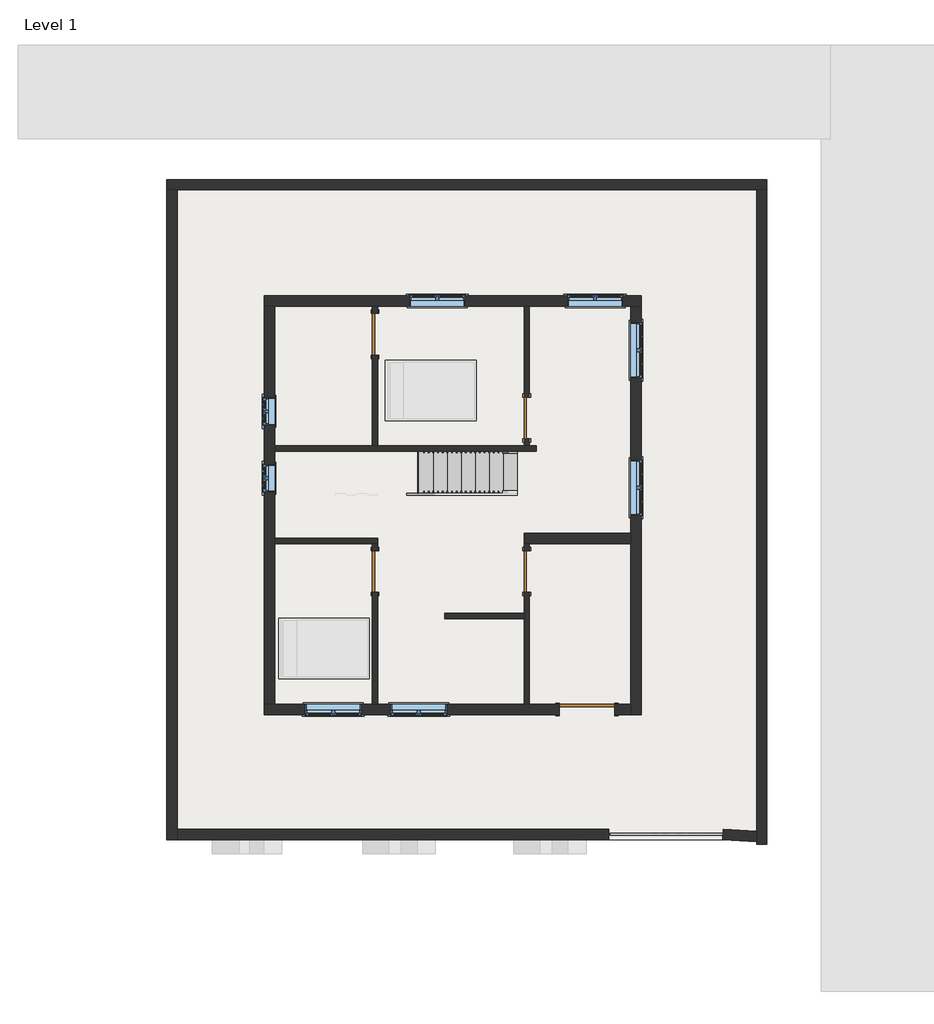
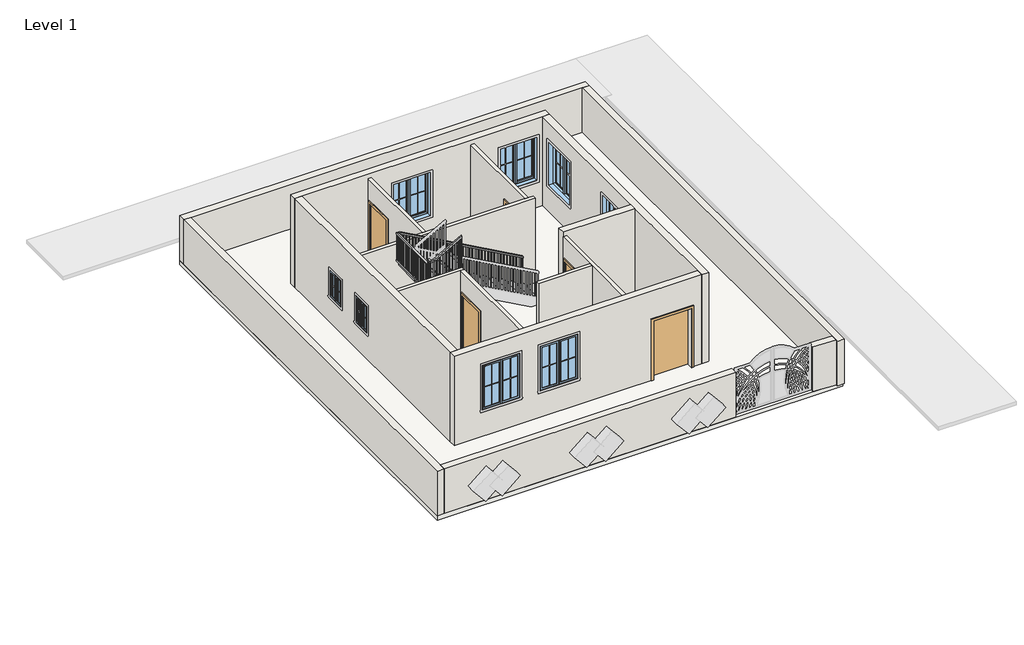
# One storey, part 1 of 2: 17 walls, 8 windows, 5 doors, 1 railing, 1 slab, 1 stair flight.
"""IFC4 building model written with IfcOpenShell, lengths in millimetres."""

from ifc_helpers import new_model, si_unit, frame, origin, origin_with_axes, place, context, project, spatial, polyline, outline, extrude, faceted_brep, transform, mapped, element, save
from components import door_e5f9f3c4, door_305aa2a5, door_48acaae4, stair_flight_91c59d30, window_c417fced, window_8377141f

model = new_model("IFC4")

# Units and contexts
model_context = context("Model", 3, world=origin())
ifc_project = project(units=[si_unit("LENGTHUNIT", "METRE", prefix="MILLI")], contexts=[model_context])

# Site, building, storey
site = spatial("IfcSite", under=ifc_project)
building = spatial("IfcBuilding", under=site)
storey = spatial("IfcBuildingStorey", under=building, Name="Level 1", Elevation=0.0)

# Doors
placement = place(None, origin())
door_shape = door_e5f9f3c4(model_context)
element("IfcDoor", 1, ObjectType="Single-Flush : 36\" x 84\"", at=placement, inside=storey, context=model_context, shape_type="MappedRepresentation", body=[
    mapped(door_shape, transform((3689.35, 13938.7372886, 0.0), x_axis=(0.0, 1.0, 0.0), y_axis=(-1.0, 0.0, 0.0), z_axis=(0.0, 0.0, 1.0))),
])
door_2_shape = door_305aa2a5(model_context)
element("IfcDoor", 2, ObjectType="Single-Flush : 36\" x 84\"", at=placement, inside=storey, context=model_context, shape_type="MappedRepresentation", body=[
    mapped(door_2_shape, transform((7004.05, 12109.9372886, 0.0), x_axis=(0.0, -1.0, 0.0), y_axis=(1.0, 0.0, 0.0), z_axis=(0.0, 0.0, 1.0))),
])
element("IfcDoor", 3, ObjectType="Single-Flush : 36\" x 84\"", at=placement, inside=storey, context=model_context, shape_type="MappedRepresentation", body=[
    mapped(door_2_shape, transform((3689.3519847, 8757.1372886, 0.0), x_axis=(0.0, -1.0, 0.0), y_axis=(1.0, 0.0, 0.0), z_axis=(0.0, 0.0, 1.0))),
])
element("IfcDoor", 4, ObjectType="Single-Flush : 36\" x 84\"", at=placement, inside=storey, context=model_context, shape_type="MappedRepresentation", body=[
    mapped(door_2_shape, transform((7004.05, 8757.1372886, 0.0), x_axis=(0.0, -1.0, 0.0), y_axis=(1.0, 0.0, 0.0), z_axis=(0.0, 0.0, 1.0))),
])
door_3_shape = door_48acaae4(model_context)
element("IfcDoor", 5, ObjectType="Single-Flush : 48\" x 80\"", at=placement, inside=storey, context=model_context, shape_type="MappedRepresentation", body=[
    mapped(door_3_shape, transform((8318.5, 5747.2372886, 0.0), x_axis=(1.0, 0.0, 0.0), y_axis=(0.0, 1.0, 0.0), z_axis=(0.0, 0.0, 1.0))),
])

# Railing
element("IfcRailing", 6, ObjectType="Handrail - Rectangular", at=placement, inside=storey, context=model_context, shape_type="SolidModel", body=[
    faceted_brep([(6794.5, 11335.2372886, 1083.7333333), (6794.5, 11335.2372886, 1025.620221), (6794.5, 11386.0372886, 1025.620221), (6794.5, 11386.0372886, 1083.7333333), (2832.1, 11335.2372886, 3285.0666667), (2818.9363978, 11335.2372886, 3234.2666667), (2818.9363978, 11386.0372886, 3234.2666667), (2832.1, 11386.0372886, 3285.0666667), (2768.6, 11335.2372886, 3285.0666667), (2768.6, 11335.2372886, 3234.2666667), (2717.8, 11386.0372886, 3234.2666667), (2717.8, 11386.0372886, 3285.0666667), (2768.6, 9608.0372886, 3285.0666667), (2768.6, 9557.2372886, 3234.2666667), (2717.8, 9557.2372886, 3234.2666667), (2717.8, 9608.0372886, 3285.0666667), (2768.6, 9608.0372886, 3461.4555402), (2768.6, 9557.2372886, 3410.6555402), (2717.8, 9557.2372886, 3410.6555402), (2717.8, 9608.0372886, 3461.4555402), (2768.6, 9531.8372886, 3461.4555402), (2768.6, 9531.8372886, 3410.6555402), (2717.8, 9481.0372886, 3410.6555402), (2717.8, 9481.0372886, 3461.4555402), (2844.8, 9531.8372886, 3461.4555402), (2857.9635773, 9531.8372886, 3410.6555402), (2857.9635773, 9481.0372886, 3410.6555402), (2844.8, 9481.0372886, 3461.4555402), (3746.5019847, 9531.8372886, 3962.4), (3746.5019847, 9481.0372886, 3962.4), (3746.5019847, 9481.0372886, 3904.2869174), (3746.5019847, 9531.8372886, 3904.2869174)], [[[0, 1, 2, 3]], [[1, 0, 4, 5]], [[2, 1, 5, 6]], [[3, 2, 6, 7]], [[0, 3, 7, 4]], [[5, 4, 8, 9]], [[6, 5, 9, 10]], [[7, 6, 10, 11]], [[4, 7, 11, 8]], [[9, 8, 12, 13]], [[10, 9, 13, 14]], [[11, 10, 14, 15]], [[8, 11, 15, 12]], [[13, 12, 16, 17]], [[14, 13, 17, 18]], [[15, 14, 18, 19]], [[12, 15, 19, 16]], [[17, 16, 20, 21]], [[18, 17, 21, 22]], [[19, 18, 22, 23]], [[16, 19, 23, 20]], [[21, 20, 24, 25]], [[22, 21, 25, 26]], [[23, 22, 26, 27]], [[20, 23, 27, 24]], [[28, 29, 30, 31]], [[25, 24, 28, 31]], [[26, 25, 31, 30]], [[27, 26, 30, 29]], [[24, 27, 29, 28]]]),
    extrude(outline(polyline([(3860.1894234, 3667.125), (3849.606113, 3648.075), (2878.6666667, 3648.075), (2878.6666667, 3667.125), (3860.1894234, 3667.125)])), frame((0.0, 9496.9122886, 0.0), z_axis=(0.0, 1.0, 0.0), x_axis=(0.0, 0.0, 1.0)), (0.0, 0.0, 1.0), 19.05),
    extrude(outline(polyline([(3803.7451014, 3565.525), (3793.1617911, 3546.475), (2878.6666667, 3546.475), (2878.6666667, 3565.525), (3803.7451014, 3565.525)])), frame((0.0, 9496.9122886, 0.0), z_axis=(0.0, 1.0, 0.0), x_axis=(0.0, 0.0, 1.0)), (0.0, 0.0, 1.0), 19.05),
    extrude(outline(polyline([(3747.3007795, 3463.925), (3736.7174691, 3444.875), (2878.6666667, 3444.875), (2878.6666667, 3463.925), (3747.3007795, 3463.925)])), frame((0.0, 9496.9122886, 0.0), z_axis=(0.0, 1.0, 0.0), x_axis=(0.0, 0.0, 1.0)), (0.0, 0.0, 1.0), 19.05),
    extrude(outline(polyline([(3690.85609, 3362.325), (3680.2727797, 3343.275), (2709.3333333, 3343.275), (2709.3333333, 3362.325), (3690.85609, 3362.325)])), frame((0.0, 9496.9122886, 0.0), z_axis=(0.0, 1.0, 0.0), x_axis=(0.0, 0.0, 1.0)), (0.0, 0.0, 1.0), 19.05),
    extrude(outline(polyline([(3634.4117681, 3260.725), (3623.8284577, 3241.675), (2709.3333333, 3241.675), (2709.3333333, 3260.725), (3634.4117681, 3260.725)])), frame((0.0, 9496.9122886, 0.0), z_axis=(0.0, 1.0, 0.0), x_axis=(0.0, 0.0, 1.0)), (0.0, 0.0, 1.0), 19.05),
    extrude(outline(polyline([(3577.9674462, 3159.125), (3567.3841358, 3140.075), (2709.3333333, 3140.075), (2709.3333333, 3159.125), (3577.9674462, 3159.125)])), frame((0.0, 9496.9122886, 0.0), z_axis=(0.0, 1.0, 0.0), x_axis=(0.0, 0.0, 1.0)), (0.0, 0.0, 1.0), 19.05),
    extrude(outline(polyline([(3521.5227567, 3057.525), (3510.9394463, 3038.475), (2540.0, 3038.475), (2540.0, 3057.525), (3521.5227567, 3057.525)])), frame((0.0, 9496.9122886, 0.0), z_axis=(0.0, 1.0, 0.0), x_axis=(0.0, 0.0, 1.0)), (0.0, 0.0, 1.0), 19.05),
    extrude(outline(polyline([(3465.0784348, 2955.925), (3454.4951244, 2936.875), (2540.0, 2936.875), (2540.0, 2955.925), (3465.0784348, 2955.925)])), frame((0.0, 9496.9122886, 0.0), z_axis=(0.0, 1.0, 0.0), x_axis=(0.0, 0.0, 1.0)), (0.0, 0.0, 1.0), 19.05),
    extrude(outline(polyline([(3408.6341128, 2854.325), (3398.0508025, 2835.275), (2540.0, 2835.275), (2540.0, 2854.325), (3408.6341128, 2854.325)])), frame((0.0, 9496.9122886, 0.0), z_axis=(0.0, 1.0, 0.0), x_axis=(0.0, 0.0, 1.0)), (0.0, 0.0, 1.0), 19.05),
    extrude(outline(polyline([(2733.675, 9541.3622886), (2752.725, 9541.3622886), (2752.725, 9522.3122886), (2733.675, 9522.3122886), (2733.675, 9541.3622886)])), frame((0.0, 0.0, 2370.6666667), z_axis=(0.0, 0.0, 1.0), x_axis=(1.0, 0.0, 0.0)), (0.0, 0.0, 1.0), 1039.9888736),
    extrude(outline(polyline([(2733.675, 9642.9622886), (2752.725, 9642.9622886), (2752.725, 9623.9122886), (2733.675, 9623.9122886), (2733.675, 9642.9622886)])), frame((0.0, 0.0, 2370.6666667), z_axis=(0.0, 0.0, 1.0), x_axis=(1.0, 0.0, 0.0)), (0.0, 0.0, 1.0), 863.6),
    extrude(outline(polyline([(2733.675, 9744.5622886), (2752.725, 9744.5622886), (2752.725, 9725.5122886), (2733.675, 9725.5122886), (2733.675, 9744.5622886)])), frame((0.0, 0.0, 2370.6666667), z_axis=(0.0, 0.0, 1.0), x_axis=(1.0, 0.0, 0.0)), (0.0, 0.0, 1.0), 863.6),
    extrude(outline(polyline([(2733.675, 9846.1622886), (2752.725, 9846.1622886), (2752.725, 9827.1122886), (2733.675, 9827.1122886), (2733.675, 9846.1622886)])), frame((0.0, 0.0, 2370.6666667), z_axis=(0.0, 0.0, 1.0), x_axis=(1.0, 0.0, 0.0)), (0.0, 0.0, 1.0), 863.6),
    extrude(outline(polyline([(2733.675, 9947.7622886), (2752.725, 9947.7622886), (2752.725, 9928.7122886), (2733.675, 9928.7122886), (2733.675, 9947.7622886)])), frame((0.0, 0.0, 2370.6666667), z_axis=(0.0, 0.0, 1.0), x_axis=(1.0, 0.0, 0.0)), (0.0, 0.0, 1.0), 863.6),
    extrude(outline(polyline([(2733.675, 10049.3622886), (2752.725, 10049.3622886), (2752.725, 10030.3122886), (2733.675, 10030.3122886), (2733.675, 10049.3622886)])), frame((0.0, 0.0, 2370.6666667), z_axis=(0.0, 0.0, 1.0), x_axis=(1.0, 0.0, 0.0)), (0.0, 0.0, 1.0), 863.6),
    extrude(outline(polyline([(2733.675, 10150.9622886), (2752.725, 10150.9622886), (2752.725, 10131.9122886), (2733.675, 10131.9122886), (2733.675, 10150.9622886)])), frame((0.0, 0.0, 2370.6666667), z_axis=(0.0, 0.0, 1.0), x_axis=(1.0, 0.0, 0.0)), (0.0, 0.0, 1.0), 863.6),
    extrude(outline(polyline([(2733.675, 10252.5622886), (2752.725, 10252.5622886), (2752.725, 10233.5122886), (2733.675, 10233.5122886), (2733.675, 10252.5622886)])), frame((0.0, 0.0, 2370.6666667), z_axis=(0.0, 0.0, 1.0), x_axis=(1.0, 0.0, 0.0)), (0.0, 0.0, 1.0), 863.6),
    extrude(outline(polyline([(2733.675, 10354.1622886), (2752.725, 10354.1622886), (2752.725, 10335.1122886), (2733.675, 10335.1122886), (2733.675, 10354.1622886)])), frame((0.0, 0.0, 2370.6666667), z_axis=(0.0, 0.0, 1.0), x_axis=(1.0, 0.0, 0.0)), (0.0, 0.0, 1.0), 863.6),
    extrude(outline(polyline([(2733.675, 10455.7622886), (2752.725, 10455.7622886), (2752.725, 10436.7122886), (2733.675, 10436.7122886), (2733.675, 10455.7622886)])), frame((0.0, 0.0, 2370.6666667), z_axis=(0.0, 0.0, 1.0), x_axis=(1.0, 0.0, 0.0)), (0.0, 0.0, 1.0), 863.6),
    extrude(outline(polyline([(2733.675, 10557.3622886), (2752.725, 10557.3622886), (2752.725, 10538.3122886), (2733.675, 10538.3122886), (2733.675, 10557.3622886)])), frame((0.0, 0.0, 2370.6666667), z_axis=(0.0, 0.0, 1.0), x_axis=(1.0, 0.0, 0.0)), (0.0, 0.0, 1.0), 863.6),
    extrude(outline(polyline([(2733.675, 10658.9622886), (2752.725, 10658.9622886), (2752.725, 10639.9122886), (2733.675, 10639.9122886), (2733.675, 10658.9622886)])), frame((0.0, 0.0, 2370.6666667), z_axis=(0.0, 0.0, 1.0), x_axis=(1.0, 0.0, 0.0)), (0.0, 0.0, 1.0), 863.6),
    extrude(outline(polyline([(2733.675, 10760.5622886), (2752.725, 10760.5622886), (2752.725, 10741.5122886), (2733.675, 10741.5122886), (2733.675, 10760.5622886)])), frame((0.0, 0.0, 2370.6666667), z_axis=(0.0, 0.0, 1.0), x_axis=(1.0, 0.0, 0.0)), (0.0, 0.0, 1.0), 863.6),
    extrude(outline(polyline([(2733.675, 10862.1622886), (2752.725, 10862.1622886), (2752.725, 10843.1122886), (2733.675, 10843.1122886), (2733.675, 10862.1622886)])), frame((0.0, 0.0, 2370.6666667), z_axis=(0.0, 0.0, 1.0), x_axis=(1.0, 0.0, 0.0)), (0.0, 0.0, 1.0), 863.6),
    extrude(outline(polyline([(2733.675, 10963.7622886), (2752.725, 10963.7622886), (2752.725, 10944.7122886), (2733.675, 10944.7122886), (2733.675, 10963.7622886)])), frame((0.0, 0.0, 2370.6666667), z_axis=(0.0, 0.0, 1.0), x_axis=(1.0, 0.0, 0.0)), (0.0, 0.0, 1.0), 863.6),
    extrude(outline(polyline([(2733.675, 11065.3622886), (2752.725, 11065.3622886), (2752.725, 11046.3122886), (2733.675, 11046.3122886), (2733.675, 11065.3622886)])), frame((0.0, 0.0, 2370.6666667), z_axis=(0.0, 0.0, 1.0), x_axis=(1.0, 0.0, 0.0)), (0.0, 0.0, 1.0), 863.6),
    extrude(outline(polyline([(2733.675, 11166.9622886), (2752.725, 11166.9622886), (2752.725, 11147.9122886), (2733.675, 11147.9122886), (2733.675, 11166.9622886)])), frame((0.0, 0.0, 2370.6666667), z_axis=(0.0, 0.0, 1.0), x_axis=(1.0, 0.0, 0.0)), (0.0, 0.0, 1.0), 863.6),
    extrude(outline(polyline([(2733.675, 11268.5622886), (2752.725, 11268.5622886), (2752.725, 11249.5122886), (2733.675, 11249.5122886), (2733.675, 11268.5622886)])), frame((0.0, 0.0, 2370.6666667), z_axis=(0.0, 0.0, 1.0), x_axis=(1.0, 0.0, 0.0)), (0.0, 0.0, 1.0), 863.6),
    extrude(outline(polyline([(3221.6618876, 2841.625), (3232.245221, 2822.575), (2370.6666667, 2822.575), (2370.6666667, 2841.625), (3221.6618876, 2841.625)])), frame((0.0, 11351.1122886, 0.0), z_axis=(0.0, 1.0, 0.0), x_axis=(0.0, 0.0, 1.0)), (0.0, 0.0, 1.0), 19.05),
    extrude(outline(polyline([(3165.2174432, 2943.225), (3175.8007765, 2924.175), (2201.3333333, 2924.175), (2201.3333333, 2943.225), (3165.2174432, 2943.225)])), frame((0.0, 11351.1122886, 0.0), z_axis=(0.0, 1.0, 0.0), x_axis=(0.0, 0.0, 1.0)), (0.0, 0.0, 1.0), 19.05),
    extrude(outline(polyline([(3108.7729988, 3044.825), (3119.3563321, 3025.775), (2201.3333333, 3025.775), (2201.3333333, 3044.825), (3108.7729988, 3044.825)])), frame((0.0, 11351.1122886, 0.0), z_axis=(0.0, 1.0, 0.0), x_axis=(0.0, 0.0, 1.0)), (0.0, 0.0, 1.0), 19.05),
    extrude(outline(polyline([(3052.3285543, 3146.425), (3062.9118876, 3127.375), (2201.3333333, 3127.375), (2201.3333333, 3146.425), (3052.3285543, 3146.425)])), frame((0.0, 11351.1122886, 0.0), z_axis=(0.0, 1.0, 0.0), x_axis=(0.0, 0.0, 1.0)), (0.0, 0.0, 1.0), 19.05),
    extrude(outline(polyline([(2995.8841099, 3248.025), (3006.4674432, 3228.975), (2032.0, 3228.975), (2032.0, 3248.025), (2995.8841099, 3248.025)])), frame((0.0, 11351.1122886, 0.0), z_axis=(0.0, 1.0, 0.0), x_axis=(0.0, 0.0, 1.0)), (0.0, 0.0, 1.0), 19.05),
    extrude(outline(polyline([(2939.4396654, 3349.625), (2950.0229988, 3330.575), (2032.0, 3330.575), (2032.0, 3349.625), (2939.4396654, 3349.625)])), frame((0.0, 11351.1122886, 0.0), z_axis=(0.0, 1.0, 0.0), x_axis=(0.0, 0.0, 1.0)), (0.0, 0.0, 1.0), 19.05),
    extrude(outline(polyline([(2882.995221, 3451.225), (2893.5785543, 3432.175), (2032.0, 3432.175), (2032.0, 3451.225), (2882.995221, 3451.225)])), frame((0.0, 11351.1122886, 0.0), z_axis=(0.0, 1.0, 0.0), x_axis=(0.0, 0.0, 1.0)), (0.0, 0.0, 1.0), 19.05),
    extrude(outline(polyline([(2826.5507765, 3552.825), (2837.1341099, 3533.775), (1862.6666667, 3533.775), (1862.6666667, 3552.825), (2826.5507765, 3552.825)])), frame((0.0, 11351.1122886, 0.0), z_axis=(0.0, 1.0, 0.0), x_axis=(0.0, 0.0, 1.0)), (0.0, 0.0, 1.0), 19.05),
    extrude(outline(polyline([(2770.1063321, 3654.425), (2780.6896654, 3635.375), (1862.6666667, 3635.375), (1862.6666667, 3654.425), (2770.1063321, 3654.425)])), frame((0.0, 11351.1122886, 0.0), z_axis=(0.0, 1.0, 0.0), x_axis=(0.0, 0.0, 1.0)), (0.0, 0.0, 1.0), 19.05),
    extrude(outline(polyline([(2713.6618876, 3756.025), (2724.245221, 3736.975), (1862.6666667, 3736.975), (1862.6666667, 3756.025), (2713.6618876, 3756.025)])), frame((0.0, 11351.1122886, 0.0), z_axis=(0.0, 1.0, 0.0), x_axis=(0.0, 0.0, 1.0)), (0.0, 0.0, 1.0), 19.05),
    extrude(outline(polyline([(2657.2174432, 3857.625), (2667.8007765, 3838.575), (1693.3333333, 3838.575), (1693.3333333, 3857.625), (2657.2174432, 3857.625)])), frame((0.0, 11351.1122886, 0.0), z_axis=(0.0, 1.0, 0.0), x_axis=(0.0, 0.0, 1.0)), (0.0, 0.0, 1.0), 19.05),
    extrude(outline(polyline([(2600.7729988, 3959.225), (2611.3563321, 3940.175), (1693.3333333, 3940.175), (1693.3333333, 3959.225), (2600.7729988, 3959.225)])), frame((0.0, 11351.1122886, 0.0), z_axis=(0.0, 1.0, 0.0), x_axis=(0.0, 0.0, 1.0)), (0.0, 0.0, 1.0), 19.05),
    extrude(outline(polyline([(2544.3285543, 4060.825), (2554.9118876, 4041.775), (1693.3333333, 4041.775), (1693.3333333, 4060.825), (2544.3285543, 4060.825)])), frame((0.0, 11351.1122886, 0.0), z_axis=(0.0, 1.0, 0.0), x_axis=(0.0, 0.0, 1.0)), (0.0, 0.0, 1.0), 19.05),
    extrude(outline(polyline([(2487.8841099, 4162.425), (2498.4674432, 4143.375), (1524.0, 4143.375), (1524.0, 4162.425), (2487.8841099, 4162.425)])), frame((0.0, 11351.1122886, 0.0), z_axis=(0.0, 1.0, 0.0), x_axis=(0.0, 0.0, 1.0)), (0.0, 0.0, 1.0), 19.05),
    extrude(outline(polyline([(2431.4396654, 4264.025), (2442.0229988, 4244.975), (1524.0, 4244.975), (1524.0, 4264.025), (2431.4396654, 4264.025)])), frame((0.0, 11351.1122886, 0.0), z_axis=(0.0, 1.0, 0.0), x_axis=(0.0, 0.0, 1.0)), (0.0, 0.0, 1.0), 19.05),
    extrude(outline(polyline([(2374.995221, 4365.625), (2385.5785543, 4346.575), (1524.0, 4346.575), (1524.0, 4365.625), (2374.995221, 4365.625)])), frame((0.0, 11351.1122886, 0.0), z_axis=(0.0, 1.0, 0.0), x_axis=(0.0, 0.0, 1.0)), (0.0, 0.0, 1.0), 19.05),
    extrude(outline(polyline([(2318.5507765, 4467.225), (2329.1341099, 4448.175), (1354.6666667, 4448.175), (1354.6666667, 4467.225), (2318.5507765, 4467.225)])), frame((0.0, 11351.1122886, 0.0), z_axis=(0.0, 1.0, 0.0), x_axis=(0.0, 0.0, 1.0)), (0.0, 0.0, 1.0), 19.05),
    extrude(outline(polyline([(2262.1063321, 4568.825), (2272.6896654, 4549.775), (1354.6666667, 4549.775), (1354.6666667, 4568.825), (2262.1063321, 4568.825)])), frame((0.0, 11351.1122886, 0.0), z_axis=(0.0, 1.0, 0.0), x_axis=(0.0, 0.0, 1.0)), (0.0, 0.0, 1.0), 19.05),
    extrude(outline(polyline([(2205.6618876, 4670.425), (2216.245221, 4651.375), (1354.6666667, 4651.375), (1354.6666667, 4670.425), (2205.6618876, 4670.425)])), frame((0.0, 11351.1122886, 0.0), z_axis=(0.0, 1.0, 0.0), x_axis=(0.0, 0.0, 1.0)), (0.0, 0.0, 1.0), 19.05),
    extrude(outline(polyline([(2149.2174432, 4772.025), (2159.8007765, 4752.975), (1185.3333333, 4752.975), (1185.3333333, 4772.025), (2149.2174432, 4772.025)])), frame((0.0, 11351.1122886, 0.0), z_axis=(0.0, 1.0, 0.0), x_axis=(0.0, 0.0, 1.0)), (0.0, 0.0, 1.0), 19.05),
    extrude(outline(polyline([(2092.7729988, 4873.625), (2103.3563321, 4854.575), (1185.3333333, 4854.575), (1185.3333333, 4873.625), (2092.7729988, 4873.625)])), frame((0.0, 11351.1122886, 0.0), z_axis=(0.0, 1.0, 0.0), x_axis=(0.0, 0.0, 1.0)), (0.0, 0.0, 1.0), 19.05),
    extrude(outline(polyline([(2036.3285543, 4975.225), (2046.9118876, 4956.175), (1185.3333333, 4956.175), (1185.3333333, 4975.225), (2036.3285543, 4975.225)])), frame((0.0, 11351.1122886, 0.0), z_axis=(0.0, 1.0, 0.0), x_axis=(0.0, 0.0, 1.0)), (0.0, 0.0, 1.0), 19.05),
    extrude(outline(polyline([(1979.8841099, 5076.825), (1990.4674432, 5057.775), (1016.0, 5057.775), (1016.0, 5076.825), (1979.8841099, 5076.825)])), frame((0.0, 11351.1122886, 0.0), z_axis=(0.0, 1.0, 0.0), x_axis=(0.0, 0.0, 1.0)), (0.0, 0.0, 1.0), 19.05),
    extrude(outline(polyline([(1923.4396654, 5178.425), (1934.0229988, 5159.375), (1016.0, 5159.375), (1016.0, 5178.425), (1923.4396654, 5178.425)])), frame((0.0, 11351.1122886, 0.0), z_axis=(0.0, 1.0, 0.0), x_axis=(0.0, 0.0, 1.0)), (0.0, 0.0, 1.0), 19.05),
    extrude(outline(polyline([(1866.995221, 5280.025), (1877.5785543, 5260.975), (1016.0, 5260.975), (1016.0, 5280.025), (1866.995221, 5280.025)])), frame((0.0, 11351.1122886, 0.0), z_axis=(0.0, 1.0, 0.0), x_axis=(0.0, 0.0, 1.0)), (0.0, 0.0, 1.0), 19.05),
    extrude(outline(polyline([(1810.5507765, 5381.625), (1821.1341099, 5362.575), (846.6666667, 5362.575), (846.6666667, 5381.625), (1810.5507765, 5381.625)])), frame((0.0, 11351.1122886, 0.0), z_axis=(0.0, 1.0, 0.0), x_axis=(0.0, 0.0, 1.0)), (0.0, 0.0, 1.0), 19.05),
    extrude(outline(polyline([(1754.1063321, 5483.225), (1764.6896654, 5464.175), (846.6666667, 5464.175), (846.6666667, 5483.225), (1754.1063321, 5483.225)])), frame((0.0, 11351.1122886, 0.0), z_axis=(0.0, 1.0, 0.0), x_axis=(0.0, 0.0, 1.0)), (0.0, 0.0, 1.0), 19.05),
    extrude(outline(polyline([(1697.6618876, 5584.825), (1708.245221, 5565.775), (846.6666667, 5565.775), (846.6666667, 5584.825), (1697.6618876, 5584.825)])), frame((0.0, 11351.1122886, 0.0), z_axis=(0.0, 1.0, 0.0), x_axis=(0.0, 0.0, 1.0)), (0.0, 0.0, 1.0), 19.05),
    extrude(outline(polyline([(1641.2174432, 5686.425), (1651.8007765, 5667.375), (677.3333333, 5667.375), (677.3333333, 5686.425), (1641.2174432, 5686.425)])), frame((0.0, 11351.1122886, 0.0), z_axis=(0.0, 1.0, 0.0), x_axis=(0.0, 0.0, 1.0)), (0.0, 0.0, 1.0), 19.05),
    extrude(outline(polyline([(1584.7729988, 5788.025), (1595.3563321, 5768.975), (677.3333333, 5768.975), (677.3333333, 5788.025), (1584.7729988, 5788.025)])), frame((0.0, 11351.1122886, 0.0), z_axis=(0.0, 1.0, 0.0), x_axis=(0.0, 0.0, 1.0)), (0.0, 0.0, 1.0), 19.05),
    extrude(outline(polyline([(1528.3285543, 5889.625), (1538.9118876, 5870.575), (677.3333333, 5870.575), (677.3333333, 5889.625), (1528.3285543, 5889.625)])), frame((0.0, 11351.1122886, 0.0), z_axis=(0.0, 1.0, 0.0), x_axis=(0.0, 0.0, 1.0)), (0.0, 0.0, 1.0), 19.05),
    extrude(outline(polyline([(1471.8841099, 5991.225), (1482.4674432, 5972.175), (508.0, 5972.175), (508.0, 5991.225), (1471.8841099, 5991.225)])), frame((0.0, 11351.1122886, 0.0), z_axis=(0.0, 1.0, 0.0), x_axis=(0.0, 0.0, 1.0)), (0.0, 0.0, 1.0), 19.05),
    extrude(outline(polyline([(1415.4396654, 6092.825), (1426.0229988, 6073.775), (508.0, 6073.775), (508.0, 6092.825), (1415.4396654, 6092.825)])), frame((0.0, 11351.1122886, 0.0), z_axis=(0.0, 1.0, 0.0), x_axis=(0.0, 0.0, 1.0)), (0.0, 0.0, 1.0), 19.05),
    extrude(outline(polyline([(1358.995221, 6194.425), (1369.5785543, 6175.375), (508.0, 6175.375), (508.0, 6194.425), (1358.995221, 6194.425)])), frame((0.0, 11351.1122886, 0.0), z_axis=(0.0, 1.0, 0.0), x_axis=(0.0, 0.0, 1.0)), (0.0, 0.0, 1.0), 19.05),
    extrude(outline(polyline([(1302.5507765, 6296.025), (1313.1341099, 6276.975), (338.6666667, 6276.975), (338.6666667, 6296.025), (1302.5507765, 6296.025)])), frame((0.0, 11351.1122886, 0.0), z_axis=(0.0, 1.0, 0.0), x_axis=(0.0, 0.0, 1.0)), (0.0, 0.0, 1.0), 19.05),
    extrude(outline(polyline([(1246.1063321, 6397.625), (1256.6896654, 6378.575), (338.6666667, 6378.575), (338.6666667, 6397.625), (1246.1063321, 6397.625)])), frame((0.0, 11351.1122886, 0.0), z_axis=(0.0, 1.0, 0.0), x_axis=(0.0, 0.0, 1.0)), (0.0, 0.0, 1.0), 19.05),
    extrude(outline(polyline([(1189.6618876, 6499.225), (1200.245221, 6480.175), (338.6666667, 6480.175), (338.6666667, 6499.225), (1189.6618876, 6499.225)])), frame((0.0, 11351.1122886, 0.0), z_axis=(0.0, 1.0, 0.0), x_axis=(0.0, 0.0, 1.0)), (0.0, 0.0, 1.0), 19.05),
    extrude(outline(polyline([(1133.2174432, 6600.825), (1143.8007765, 6581.775), (169.3333333, 6581.775), (169.3333333, 6600.825), (1133.2174432, 6600.825)])), frame((0.0, 11351.1122886, 0.0), z_axis=(0.0, 1.0, 0.0), x_axis=(0.0, 0.0, 1.0)), (0.0, 0.0, 1.0), 19.05),
    extrude(outline(polyline([(1076.7729988, 6702.425), (1087.3563321, 6683.375), (169.3333333, 6683.375), (169.3333333, 6702.425), (1076.7729988, 6702.425)])), frame((0.0, 11351.1122886, 0.0), z_axis=(0.0, 1.0, 0.0), x_axis=(0.0, 0.0, 1.0)), (0.0, 0.0, 1.0), 19.05),
    extrude(outline(polyline([(2733.675, 9515.9622886), (2752.725, 9515.9622886), (2752.725, 9496.9122886), (2733.675, 9496.9122886), (2733.675, 9515.9622886)])), frame((0.0, 0.0, 2370.6666667), z_axis=(0.0, 0.0, 1.0), x_axis=(1.0, 0.0, 0.0)), (0.0, 0.0, 1.0), 1039.9888736),
    extrude(outline(polyline([(2752.725, 11370.1622886), (2752.725, 11351.1122886), (2733.675, 11351.1122886), (2733.675, 11370.1622886), (2752.725, 11370.1622886)])), frame((0.0, 0.0, 2370.6666667), z_axis=(0.0, 0.0, 1.0), x_axis=(1.0, 0.0, 0.0)), (0.0, 0.0, 1.0), 863.6),
    extrude(outline(polyline([(3904.2869174, 3746.5019847), (3893.703607, 3727.4519847), (2878.6666667, 3727.4519847), (2878.6666667, 3746.5019847), (3904.2869174, 3746.5019847)])), frame((0.0, 9496.9122886, 0.0), z_axis=(0.0, 1.0, 0.0), x_axis=(0.0, 0.0, 1.0)), (0.0, 0.0, 1.0), 19.05),
    extrude(outline(polyline([(1025.620221, 6794.5), (1036.2035543, 6775.45), (169.3333333, 6775.45), (169.3333333, 6794.5), (1025.620221, 6794.5)])), frame((0.0, 11351.1122886, 0.0), z_axis=(0.0, 1.0, 0.0), x_axis=(0.0, 0.0, 1.0)), (0.0, 0.0, 1.0), 19.05),
])

# Slab
element("IfcSlab", 7, ObjectType="Generic - 12\"", at=placement, inside=storey, context=model_context, shape_type="SweptSolid", body=[
    extrude(outline(polyline([(12249.1058463, 17315.367514), (12249.1058463, 2902.4372886), (-857.2941537, 2902.4372886), (-857.2941537, 17315.367514), (12249.1058463, 17315.367514)])), frame((0.0, 0.0, -152.4), z_axis=(0.0, 0.0, 1.0), x_axis=(1.0, 0.0, 0.0)), (0.0, 0.0, 1.0), 152.4),
])

# Stair flight
stair_flight_shape = stair_flight_91c59d30(model_context)
element("IfcStairFlight", 8, ObjectType="2\" Tread 1\" Nosing 1/4\" Riser", at=placement, inside=storey, context=model_context, shape_type="MappedRepresentation", body=[
    mapped(stair_flight_shape, transform((0.0, 0.0, 0.0), x_axis=(1.0, 0.0, 0.0), y_axis=(0.0, 1.0, 0.0), z_axis=(0.0, 0.0, 1.0))),
])

# Walls
element("IfcWall", 9, ObjectType="Generic - 5\"", at=placement, inside=storey, context=model_context, shape_type="SweptSolid", body=[
    extrude(outline(polyline([(14548.3372886, 0.0), (14395.9372886, 0.0), (14395.9372886, 2133.6), (13481.5372886, 2133.6), (13481.5372886, 0.0), (11500.3372886, 0.0), (11500.3372886, 2895.6), (14548.3372886, 2895.6), (14548.3372886, 0.0)])), frame((3632.2, 0.0, 0.0), z_axis=(1.0, 0.0, 0.0), x_axis=(0.0, 1.0, 0.0)), (0.0, 0.0, 1.0), 114.3),
])
element("IfcWall", 10, ObjectType="Generic - 5\"", at=placement, inside=storey, context=model_context, shape_type="SweptSolid", body=[
    extrude(outline(polyline([(11652.7372886, 2133.6), (11652.7372886, 0.0), (11500.3372886, 0.0), (11500.3372886, 2895.6), (14548.3372886, 2895.6), (14548.3372886, 0.0), (12567.1372886, 0.0), (12567.1372886, 2133.6), (11652.7372886, 2133.6)])), frame((6946.9, 0.0, 0.0), z_axis=(1.0, 0.0, 0.0), x_axis=(0.0, 1.0, 0.0)), (0.0, 0.0, 1.0), 114.3),
])
element("IfcWall", 11, ObjectType="Generic - 5\"", at=placement, inside=storey, context=model_context, shape_type="Brep", body=[
    faceted_brep([(1498.6, 11386.0372886, 0.0), (7213.6, 11386.0372886, 0.0), (7213.6, 11386.0372886, 2895.6), (1498.6, 11386.0372886, 2895.6), (1498.6, 11500.3372886, 0.0), (1498.6, 11500.3372886, 2895.6), (3632.2, 11500.3372886, 2895.6), (3746.5, 11500.3372886, 2895.6), (6946.9, 11500.3372886, 2895.6), (7061.2, 11500.3372886, 2895.6), (7213.6, 11500.3372886, 2895.6), (7213.6, 11500.3372886, 0.0), (7061.2, 11500.3372886, 0.0), (6946.9, 11500.3372886, 0.0), (3746.5, 11500.3372886, 0.0), (3632.2, 11500.3372886, 0.0)], [[[0, 1, 2, 3]], [[4, 5, 6, 7, 8, 9, 10, 11, 12, 13, 14, 15]], [[1, 0, 4, 15, 14, 13, 12, 11]], [[2, 1, 11, 10]], [[0, 3, 5, 4]], [[3, 2, 10, 9, 8, 7, 6, 5]]]),
])
element("IfcWall", 12, ObjectType="Generic - 5\"", at=placement, inside=storey, context=model_context, shape_type="Brep", body=[
    faceted_brep([(1498.6, 9366.7372886, 0.0), (3632.2019847, 9366.7372886, 0.0), (3746.5019847, 9366.7372886, 0.0), (3746.5019847, 9366.7372886, 2895.6), (3632.2019847, 9366.7372886, 2895.6), (1498.6, 9366.7372886, 2895.6), (1498.6, 9481.0372886, 0.0), (1498.6, 9481.0372886, 2895.6), (3746.5019847, 9481.0372886, 2895.6), (3746.5019847, 9481.0372886, 0.0)], [[[0, 1, 2, 3, 4, 5]], [[6, 7, 8, 9]], [[2, 1, 0, 6, 9]], [[0, 5, 7, 6]], [[3, 2, 9, 8]], [[5, 4, 3, 8, 7]]]),
])
element("IfcWall", 13, ObjectType="Generic - 5\"", at=placement, inside=storey, context=model_context, shape_type="SweptSolid", body=[
    extrude(outline(polyline([(8299.9372886, 2133.6), (8299.9372886, 0.0), (5861.5372886, 0.0), (5861.5372886, 2895.6), (9366.7372886, 2895.6), (9366.7372886, 0.0), (9214.3372886, 0.0), (9214.3372886, 2133.6), (8299.9372886, 2133.6)])), frame((3632.2019847, 0.0, 0.0), z_axis=(1.0, 0.0, 0.0), x_axis=(0.0, 1.0, 0.0)), (0.0, 0.0, 1.0), 114.3),
])
element("IfcWall", 14, ObjectType="Generic - 5\"", at=placement, inside=storey, context=model_context, shape_type="Brep", body=[
    faceted_brep([(7061.2, 5861.5372886, 0.0), (7061.2, 8299.9372886, 0.0), (7061.2, 8299.9372886, 2133.6), (7061.2, 9214.3372886, 2133.6), (7061.2, 9214.3372886, 0.0), (7061.2, 9366.7372886, 0.0), (7061.2, 9366.7372886, 2895.6), (7061.2, 5861.5372886, 2895.6), (6946.9, 8299.9372886, 2133.6), (6946.9, 8299.9372886, 0.0), (6946.9, 7842.7372886, 0.0), (6946.9, 7728.4372886, 0.0), (6946.9, 5861.5372886, 0.0), (6946.9, 5861.5372886, 2895.6), (6946.9, 7728.4372886, 2895.6), (6946.9, 7842.7372886, 2895.6), (6946.9, 9366.7372886, 2895.6), (6946.9, 9366.7372886, 0.0), (6946.9, 9214.3372886, 0.0), (6946.9, 9214.3372886, 2133.6)], [[[0, 1, 2, 3, 4, 5, 6, 7]], [[8, 9, 10, 11, 12, 13, 14, 15, 16, 17, 18, 19]], [[18, 17, 5, 4]], [[12, 11, 10, 9, 1, 0]], [[0, 7, 13, 12]], [[6, 5, 17, 16]], [[2, 1, 9, 8]], [[3, 2, 8, 19]], [[4, 3, 19, 18]], [[7, 6, 16, 15, 14, 13]]]),
])
element("IfcWall", 15, ObjectType="Generic - 5\"", at=placement, inside=storey, context=model_context, shape_type="SweptSolid", body=[
    extrude(outline(polyline([(5215.2207778, 7842.7372886), (6946.9, 7842.7372886), (6946.9, 7728.4372886), (5215.2207778, 7728.4372886), (5215.2207778, 7842.7372886)])), origin_with_axes(), (0.0, 0.0, 1.0), 2895.6),
])
element("IfcWall", 16, ObjectType="Generic - 8\"", at=placement, inside=storey, context=model_context, shape_type="Brep", body=[
    faceted_brep([(1270.0, 14548.3372886, 0.0), (1498.6, 14548.3372886, 0.0), (3632.2, 14548.3372886, 0.0), (3746.5, 14548.3372886, 0.0), (6946.9, 14548.3372886, 0.0), (7061.2, 14548.3372886, 0.0), (9271.0, 14548.3372886, 0.0), (9499.6, 14548.3372886, 0.0), (9499.6, 14548.3372886, 3048.0), (9271.0, 14548.3372886, 3048.0), (1498.6, 14548.3372886, 3048.0), (1270.0, 14548.3372886, 3048.0), (9105.9, 14548.3372886, 2438.4), (9105.9, 14548.3372886, 914.4), (7886.7, 14548.3372886, 914.4), (7886.7, 14548.3372886, 2438.4), (5662.6125, 14548.3372886, 2438.4), (5662.6125, 14548.3372886, 914.4), (4443.4125, 14548.3372886, 914.4), (4443.4125, 14548.3372886, 2438.4), (1270.0, 14776.9372886, 0.0), (1270.0, 14776.9372886, 3048.0), (9499.6, 14776.9372886, 3048.0), (9499.6, 14776.9372886, 0.0), (9105.9, 14776.9372886, 2438.4), (7886.7, 14776.9372886, 2438.4), (7886.7, 14776.9372886, 914.4), (9105.9, 14776.9372886, 914.4), (5662.6125, 14776.9372886, 2438.4), (4443.4125, 14776.9372886, 2438.4), (4443.4125, 14776.9372886, 914.4), (5662.6125, 14776.9372886, 914.4)], [[[0, 1, 2, 3, 4, 5, 6, 7, 8, 9, 10, 11], [12, 13, 14, 15], [16, 17, 18, 19]], [[20, 21, 22, 23], [24, 25, 26, 27], [28, 29, 30, 31]], [[7, 6, 5, 4, 3, 2, 1, 0, 20, 23]], [[11, 10, 9, 8, 22, 21]], [[8, 7, 23, 22]], [[0, 11, 21, 20]], [[13, 12, 24, 27]], [[14, 13, 27, 26]], [[15, 14, 26, 25]], [[12, 15, 25, 24]], [[17, 16, 28, 31]], [[18, 17, 31, 30]], [[19, 18, 30, 29]], [[16, 19, 29, 28]]]),
])
element("IfcWall", 17, ObjectType="Generic - 8\"", at=placement, inside=storey, context=model_context, shape_type="Brep", body=[
    faceted_brep([(9271.0, 14548.3372886, 0.0), (9271.0, 9595.3372886, 0.0), (9271.0, 9366.7372886, 0.0), (9271.0, 5861.5372886, 0.0), (9271.0, 5632.9372886, 0.0), (9271.0, 5632.9372886, 3048.0), (9271.0, 5861.5372886, 3048.0), (9271.0, 9366.7372886, 3048.0), (9271.0, 9595.3372886, 3048.0), (9271.0, 14548.3372886, 3048.0), (9271.0, 12979.8872886, 2438.4), (9271.0, 12979.8872886, 914.4), (9271.0, 14199.0872886, 914.4), (9271.0, 14199.0872886, 2438.4), (9271.0, 9976.3372886, 2438.4), (9271.0, 9976.3372886, 914.4), (9271.0, 11195.5372886, 914.4), (9271.0, 11195.5372886, 2438.4), (9499.6, 14548.3372886, 0.0), (9499.6, 14548.3372886, 3048.0), (9499.6, 5632.9372886, 3048.0), (9499.6, 5632.9372886, 0.0), (9499.6, 12979.8872886, 2438.4), (9499.6, 14199.0872886, 2438.4), (9499.6, 14199.0872886, 914.4), (9499.6, 12979.8872886, 914.4), (9499.6, 9976.3372886, 2438.4), (9499.6, 11195.5372886, 2438.4), (9499.6, 11195.5372886, 914.4), (9499.6, 9976.3372886, 914.4)], [[[0, 1, 2, 3, 4, 5, 6, 7, 8, 9], [10, 11, 12, 13], [14, 15, 16, 17]], [[18, 19, 20, 21], [22, 23, 24, 25], [26, 27, 28, 29]], [[4, 3, 2, 1, 0, 18, 21]], [[9, 8, 7, 6, 5, 20, 19]], [[0, 9, 19, 18]], [[5, 4, 21, 20]], [[11, 10, 22, 25]], [[12, 11, 25, 24]], [[13, 12, 24, 23]], [[10, 13, 23, 22]], [[15, 14, 26, 29]], [[16, 15, 29, 28]], [[17, 16, 28, 27]], [[14, 17, 27, 26]]]),
])
element("IfcWall", 18, ObjectType="Generic - 8\"", at=placement, inside=storey, context=model_context, shape_type="Brep", body=[
    faceted_brep([(9271.0, 5861.5372886, 0.0), (8928.1, 5861.5372886, 0.0), (8928.1, 5861.5372886, 2032.0), (7708.9, 5861.5372886, 2032.0), (7708.9, 5861.5372886, 0.0), (7061.2, 5861.5372886, 0.0), (6946.9, 5861.5372886, 0.0), (3746.5019847, 5861.5372886, 0.0), (3632.2019847, 5861.5372886, 0.0), (1498.6, 5861.5372886, 0.0), (1270.0, 5861.5372886, 0.0), (1270.0, 5861.5372886, 3048.0), (1498.6, 5861.5372886, 3048.0), (9271.0, 5861.5372886, 3048.0), (4037.8082347, 5861.5372886, 2438.4), (4037.8082347, 5861.5372886, 914.4), (5257.0082347, 5861.5372886, 914.4), (5257.0082347, 5861.5372886, 2438.4), (2173.2894847, 5861.5372886, 2438.4), (2173.2894847, 5861.5372886, 914.4), (3392.4894847, 5861.5372886, 914.4), (3392.4894847, 5861.5372886, 2438.4), (8928.1, 5632.9372886, 2032.0), (8928.1, 5632.9372886, 0.0), (9271.0, 5632.9372886, 0.0), (9271.0, 5632.9372886, 3048.0), (1270.0, 5632.9372886, 3048.0), (1270.0, 5632.9372886, 0.0), (7708.9, 5632.9372886, 0.0), (7708.9, 5632.9372886, 2032.0), (4037.8082347, 5632.9372886, 2438.4), (5257.0082347, 5632.9372886, 2438.4), (5257.0082347, 5632.9372886, 914.4), (4037.8082347, 5632.9372886, 914.4), (2173.2894847, 5632.9372886, 2438.4), (3392.4894847, 5632.9372886, 2438.4), (3392.4894847, 5632.9372886, 914.4), (2173.2894847, 5632.9372886, 914.4)], [[[0, 1, 2, 3, 4, 5, 6, 7, 8, 9, 10, 11, 12, 13], [14, 15, 16, 17], [18, 19, 20, 21]], [[22, 23, 24, 25, 26, 27, 28, 29], [30, 31, 32, 33], [34, 35, 36, 37]], [[28, 27, 10, 9, 8, 7, 6, 5, 4]], [[24, 23, 1, 0]], [[13, 12, 11, 26, 25]], [[0, 13, 25, 24]], [[11, 10, 27, 26]], [[15, 14, 30, 33]], [[16, 15, 33, 32]], [[17, 16, 32, 31]], [[14, 17, 31, 30]], [[19, 18, 34, 37]], [[20, 19, 37, 36]], [[21, 20, 36, 35]], [[18, 21, 35, 34]], [[2, 1, 23, 22]], [[3, 2, 22, 29]], [[4, 3, 29, 28]]]),
])
element("IfcWall", 19, ObjectType="Generic - 8\"", at=placement, inside=storey, context=model_context, shape_type="Brep", body=[
    faceted_brep([(1498.6, 5861.5372886, 0.0), (1498.6, 9366.7372886, 0.0), (1498.6, 9481.0372886, 0.0), (1498.6, 11386.0372886, 0.0), (1498.6, 11500.3372886, 0.0), (1498.6, 14548.3372886, 0.0), (1498.6, 14548.3372886, 3048.0), (1498.6, 5861.5372886, 3048.0), (1498.6, 12557.6122886, 1828.8), (1498.6, 12557.6122886, 914.4), (1498.6, 11948.0122886, 914.4), (1498.6, 11948.0122886, 1828.8), (1498.6, 11100.2872886, 1828.8), (1498.6, 11100.2872886, 914.4), (1498.6, 10490.6872886, 914.4), (1498.6, 10490.6872886, 1828.8), (1270.0, 5861.5372886, 0.0), (1270.0, 5861.5372886, 3048.0), (1270.0, 14548.3372886, 3048.0), (1270.0, 14548.3372886, 0.0), (1270.0, 12557.6122886, 1828.8), (1270.0, 11948.0122886, 1828.8), (1270.0, 11948.0122886, 914.4), (1270.0, 12557.6122886, 914.4), (1270.0, 11100.2872886, 1828.8), (1270.0, 10490.6872886, 1828.8), (1270.0, 10490.6872886, 914.4), (1270.0, 11100.2872886, 914.4)], [[[0, 1, 2, 3, 4, 5, 6, 7], [8, 9, 10, 11], [12, 13, 14, 15]], [[16, 17, 18, 19], [20, 21, 22, 23], [24, 25, 26, 27]], [[5, 4, 3, 2, 1, 0, 16, 19]], [[7, 6, 18, 17]], [[6, 5, 19, 18]], [[0, 7, 17, 16]], [[9, 8, 20, 23]], [[10, 9, 23, 22]], [[11, 10, 22, 21]], [[8, 11, 21, 20]], [[13, 12, 24, 27]], [[14, 13, 27, 26]], [[15, 14, 26, 25]], [[12, 15, 25, 24]]]),
])
element("IfcWall", 20, ObjectType="Generic - 8\"", at=placement, inside=storey, context=model_context, shape_type="Brep", body=[
    faceted_brep([(6946.9, 9366.7372886, 0.0), (7061.2, 9366.7372886, 0.0), (9271.0, 9366.7372886, 0.0), (9271.0, 9366.7372886, 3048.0), (6946.9, 9366.7372886, 3048.0), (6946.9, 9366.7372886, 2895.6), (6946.9, 9595.3372886, 0.0), (6946.9, 9595.3372886, 3048.0), (9271.0, 9595.3372886, 3048.0), (9271.0, 9595.3372886, 0.0)], [[[0, 1, 2, 3, 4, 5]], [[6, 7, 8, 9]], [[2, 1, 0, 6, 9]], [[4, 3, 8, 7]], [[0, 5, 4, 7, 6]], [[3, 2, 9, 8]]]),
])
element("IfcWall", 21, ObjectType="Generic - 8\"", at=placement, inside=storey, context=model_context, shape_type="Brep", body=[
    faceted_brep([(-857.2941537, 17086.767514, 0.0), (-628.6941537, 17086.767514, 0.0), (12020.5058463, 17086.767514, 0.0), (12249.1058463, 17086.767514, 0.0), (12249.1058463, 17086.767514, 1524.0), (12020.5058463, 17086.767514, 1524.0), (-628.6941537, 17086.767514, 1524.0), (-857.2941537, 17086.767514, 1524.0), (-857.2941537, 17315.367514, 0.0), (-857.2941537, 17315.367514, 1524.0), (12249.1058463, 17315.367514, 1524.0), (12249.1058463, 17315.367514, 0.0)], [[[0, 1, 2, 3, 4, 5, 6, 7]], [[8, 9, 10, 11]], [[3, 2, 1, 0, 8, 11]], [[7, 6, 5, 4, 10, 9]], [[4, 3, 11, 10]], [[0, 7, 9, 8]]]),
])
element("IfcWall", 22, ObjectType="Generic - 8\"", at=placement, inside=storey, context=model_context, shape_type="Brep", body=[
    faceted_brep([(12020.5058463, 17086.767514, 0.0), (12020.5058463, 3089.4404059, 0.0), (12020.5058463, 2860.5266876, 0.0), (12020.5058463, 2799.267514, 0.0), (12020.5058463, 2799.267514, 1524.0), (12020.5058463, 2860.5266876, 1524.0), (12020.5058463, 3089.4404059, 1524.0), (12020.5058463, 17086.767514, 1524.0), (12249.1058463, 17086.767514, 0.0), (12249.1058463, 17086.767514, 1524.0), (12249.1058463, 2799.267514, 1524.0), (12249.1058463, 2799.267514, 0.0)], [[[0, 1, 2, 3, 4, 5, 6, 7]], [[8, 9, 10, 11]], [[3, 2, 1, 0, 8, 11]], [[4, 3, 11, 10]], [[7, 6, 5, 4, 10, 9]], [[0, 7, 9, 8]]]),
])
element("IfcWall", 23, ObjectType="Generic - 8\"", at=placement, inside=storey, context=model_context, shape_type="Brep", body=[
    faceted_brep([(-628.6941537, 2902.4372886, 0.0), (-628.6941537, 3131.0372886, 0.0), (-628.6941537, 17086.767514, 0.0), (-628.6941537, 17086.767514, 1524.0), (-628.6941537, 3131.0372886, 1524.0), (-628.6941537, 2902.4372886, 1524.0), (-857.2941537, 2902.4372886, 0.0), (-857.2941537, 2902.4372886, 1524.0), (-857.2941537, 17086.767514, 1524.0), (-857.2941537, 17086.767514, 0.0)], [[[0, 1, 2, 3, 4, 5]], [[6, 7, 8, 9]], [[2, 1, 0, 6, 9]], [[5, 4, 3, 8, 7]], [[3, 2, 9, 8]], [[0, 5, 7, 6]]]),
])
element("IfcWall", 24, ObjectType="Generic - 8\"", at=placement, inside=storey, context=model_context, shape_type="SweptSolid", body=[
    extrude(outline(polyline([(11296.8793306, 3127.3640646), (12020.5058463, 3089.4404059), (12020.5058463, 2860.5266876), (11284.915331, 2899.0773529), (11296.8793306, 3127.3640646)])), origin_with_axes(), (0.0, 0.0, 1.0), 1524.0),
])
element("IfcWall", 25, ObjectType="Generic - 8\"", at=placement, inside=storey, context=model_context, shape_type="SweptSolid", body=[
    extrude(outline(polyline([(-628.6941537, 3131.0372886), (8797.1491824, 3131.0372886), (8797.1491824, 2902.4372886), (-628.6941537, 2902.4372886), (-628.6941537, 3131.0372886)])), origin_with_axes(), (0.0, 0.0, 1.0), 1524.0),
])

# Windows
window_shape = window_c417fced(model_context)
element("IfcWindow", 26, ObjectType="Window-Casement-Double : 24\" x 36\"", at=placement, inside=storey, context=model_context, shape_type="MappedRepresentation", body=[
    mapped(window_shape, transform((1384.3, 12252.8122886, 0.0), x_axis=(0.0, 1.0, 0.0), y_axis=(-1.0, 0.0, 0.0), z_axis=(0.0, 0.0, 1.0))),
])
element("IfcWindow", 27, ObjectType="Window-Casement-Double : 24\" x 36\"", at=placement, inside=storey, context=model_context, shape_type="MappedRepresentation", body=[
    mapped(window_shape, transform((1384.3, 10795.4872886, 0.0), x_axis=(0.0, 1.0, 0.0), y_axis=(-1.0, 0.0, 0.0), z_axis=(0.0, 0.0, 1.0))),
])
window_2_shape = window_8377141f(model_context)
element("IfcWindow", 28, ObjectType="Window-Casement-Double : 48\" x 60\"", at=placement, inside=storey, context=model_context, shape_type="MappedRepresentation", body=[
    mapped(window_2_shape, transform((9385.3, 13589.4872886, 0.0), x_axis=(0.0, -1.0, 0.0), y_axis=(1.0, 0.0, 0.0), z_axis=(0.0, 0.0, 1.0))),
])
element("IfcWindow", 29, ObjectType="Window-Casement-Double : 48\" x 60\"", at=placement, inside=storey, context=model_context, shape_type="MappedRepresentation", body=[
    mapped(window_2_shape, transform((8496.3, 14662.6372886, 0.0), x_axis=(1.0, 0.0, 0.0), y_axis=(0.0, 1.0, 0.0), z_axis=(0.0, 0.0, 1.0))),
])
element("IfcWindow", 30, ObjectType="Window-Casement-Double : 48\" x 60\"", at=placement, inside=storey, context=model_context, shape_type="MappedRepresentation", body=[
    mapped(window_2_shape, transform((5053.0125, 14662.6372886, 0.0), x_axis=(1.0, 0.0, 0.0), y_axis=(0.0, 1.0, 0.0), z_axis=(0.0, 0.0, 1.0))),
])
element("IfcWindow", 31, ObjectType="Window-Casement-Double : 48\" x 60\"", at=placement, inside=storey, context=model_context, shape_type="MappedRepresentation", body=[
    mapped(window_2_shape, transform((9385.3, 10585.9372886, 0.0), x_axis=(0.0, -1.0, 0.0), y_axis=(1.0, 0.0, 0.0), z_axis=(0.0, 0.0, 1.0))),
])
element("IfcWindow", 32, ObjectType="Window-Casement-Double : 48\" x 60\"", at=placement, inside=storey, context=model_context, shape_type="MappedRepresentation", body=[
    mapped(window_2_shape, transform((4647.4082347, 5747.2372886, 0.0), x_axis=(-1.0, 0.0, 0.0), y_axis=(0.0, -1.0, 0.0), z_axis=(0.0, 0.0, 1.0))),
])
element("IfcWindow", 33, ObjectType="Window-Casement-Double : 48\" x 60\"", at=placement, inside=storey, context=model_context, shape_type="MappedRepresentation", body=[
    mapped(window_2_shape, transform((2782.8894847, 5747.2372886, 0.0), x_axis=(-1.0, 0.0, 0.0), y_axis=(0.0, -1.0, 0.0), z_axis=(0.0, 0.0, 1.0))),
])

save(model, "model.ifc")

# Revit data of these elements
# Type "Single-Flush : 36\" x 84\""
#   Type Mark = "1"
#   Construction Type Id = "MDOOR"
#   Assembly Code = "C1020"
#   Analytic Construction = "Metal"
#   Thickness = 0' - 2"
#   Heat Transfer Coefficient (U) = 0.651978 BTU/(h·ft²·°F)
#   Height = 7' - 0"
#   Trim Projection Ext = 0' - 1"
#   Trim Projection Int = 0' - 1"
#   Trim Width = 0' - 3"
#   Width = 3' - 0"
#   Define Thermal Properties by = 1
#   Define Thermal Properties by = 1
#   Door Material = Door - Panel
#   Frame Material = Door - Frame
#   Visual Light Transmittance = 0
#   Solar Heat Gain Coefficient = 0
#   Function = (empty or 0)
#   Wall Closure = (empty or 0)
# Type "Single-Flush : 48\" x 80\""
#   Type Mark = "5"
#   Construction Type Id = "MDOOR"
#   Assembly Code = "C1020"
#   Analytic Construction = "Metal"
#   Thickness = 0' - 2"
#   Heat Transfer Coefficient (U) = 0.651978 BTU/(h·ft²·°F)
#   Height = 6' - 8"
#   Trim Projection Ext = 0' - 1"
#   Trim Projection Int = 0' - 1"
#   Trim Width = 0' - 3"
#   Width = 4' - 0"
#   Define Thermal Properties by = 1
#   Define Thermal Properties by = 1
#   Door Material = Door - Panel
#   Frame Material = Door - Frame
#   Visual Light Transmittance = 0
#   Solar Heat Gain Coefficient = 0
#   Function = (empty or 0)
#   Wall Closure = (empty or 0)
# Type "Handrail - Rectangular"
#   Assembly Code = "C2010400"
#   built-in parameter 1008612 = 0.0416667 (stored number, unit not read)
#   built-in parameter 1008611 = 0.0416667 (stored number, unit not read)
#   built-in parameter 1008609 = 0.333333 (stored number, unit not read)
#   built-in parameter 1008604 = 0.166667 (stored number, unit not read)
#   built-in parameter 1008603 = 0.166667 (stored number, unit not read)
#   Railing Height = 3' - 0"
#   built-in parameter 1008630 = 2
#   built-in parameter 1008610 = 2
#   built-in parameter 1008618 = Baluster - Square : 3/4"
# Type "Generic - 12\""
#   Assembly Code = "B1010"
#   Function = 0
#   Layers, outside or top first: 0' - 6" no material (function 1)
# Type "Generic - 5\""
#   Assembly Code = "B2010"
#   Layers, outside or top first: 0' - 4 1/2" no material (function 1)
# Type "Generic - 8\""
#   Assembly Code = "B2010"
#   Layers, outside or top first: 0' - 9" "Softwood, Lumber" (function 1)
# Type "Window-Casement-Double : 24\" x 36\""
#   Type Mark = "14"
#   Fire Rating = "0.5h"
#   Assembly Code = "B2020100"
#   Analytic Construction = "Double glazing - domestic"
#   Frame Extension [instance default] = 0' - 0 1/4"
#   Window Inset [instance default] = 0' - 0"
#   Wall Thickness [instance default] = 0' - 6"
#   Interior Wall Closure [instance default] = 0' - 2 1/4"
#   Half Width = 1' - 0"
#   Visual Light Transmittance = 0.81
#   Thermal Resistance (R) = 1.8146 (h·ft²·°F)/BTU
#   Solar Heat Gain Coefficient = 0.76
#   Rough Width = 2' - 0 1/2"
#   Rough Height = 3' - 0 1/2"
#   Height = 3' - 0"
#   Heat Transfer Coefficient (U) = 0.5511 BTU/(h·ft²·°F)
#   Exterior Wall Closure [instance default] = 0' - 1 1/4"
#   Extension Jamb [instance default] = 0' - 2 1/4"
#   Default Sill Height = 3' - 0"
#   Width = 2' - 0"
#   Define Thermal Properties by = 0
#   Muntin Visibility = yes
#   Interior Trim Visibility [instance default] = yes
#   Exterior Trim Visibility [instance default] = yes
#   Extension Jamb Visibility [instance default] = yes
#   Interior Trim Material = Wood - Stained
#   Muntin Pattern = Muntin Pattern_2x2 : Muntin Pattern_2x2
#   Interior Trim = Trim-Window-Interior-Flat : Picture Frame
#   Interior Frame Material = Wood - Stained
#   Glass Panel Material = Glass
#   Exterior Trim Material = Clad - White
#   Exterior Trim = Trim-Window-Exterior-Flat : with Sill
#   Exterior Frame Material = Clad - White
#   Wall Closure = (empty or 0)
# Type "Window-Casement-Double : 48\" x 60\""
#   Type Mark = "17"
#   Fire Rating = "0.5h"
#   Assembly Code = "B2020100"
#   Analytic Construction = "Double glazing - domestic"
#   Frame Extension [instance default] = 0' - 0 1/4"
#   Window Inset [instance default] = 0' - 0"
#   Wall Thickness [instance default] = 0' - 6"
#   Interior Wall Closure [instance default] = 0' - 2 1/4"
#   Half Width = 2' - 0"
#   Visual Light Transmittance = 0.81
#   Thermal Resistance (R) = 1.8146 (h·ft²·°F)/BTU
#   Solar Heat Gain Coefficient = 0.76
#   Rough Width = 4' - 0 1/2"
#   Rough Height = 5' - 0 1/2"
#   Height = 5' - 0"
#   Heat Transfer Coefficient (U) = 0.5511 BTU/(h·ft²·°F)
#   Exterior Wall Closure [instance default] = 0' - 1 1/4"
#   Extension Jamb [instance default] = 0' - 2 1/4"
#   Default Sill Height = 3' - 0"
#   Width = 4' - 0"
#   Define Thermal Properties by = 0
#   Muntin Visibility = yes
#   Interior Trim Visibility [instance default] = yes
#   Exterior Trim Visibility [instance default] = yes
#   Extension Jamb Visibility [instance default] = yes
#   Interior Trim Material = Wood - Stained
#   Muntin Pattern = Muntin Pattern_2x2 : Muntin Pattern_2x2
#   Interior Trim = Trim-Window-Interior-Flat : Picture Frame
#   Interior Frame Material = Wood - Stained
#   Glass Panel Material = Glass
#   Exterior Trim Material = Clad - White
#   Exterior Trim = Trim-Window-Exterior-Flat : with Sill
#   Exterior Frame Material = Clad - White
#   Wall Closure = (empty or 0)
# Elements 1, 2, 3, 4 (IfcDoor, "Single-Flush : 36\" x 84\"")
#   Phase Created = New Construction
#   Materials on its faces: "Door - Frame", "Door - Panel"
# Element 5 (IfcDoor, "Single-Flush : 48\" x 80\"")
#   Phase Created = New Construction
#   Materials on its faces: "Door - Frame", "Door - Panel"
# Element 6 (IfcRailing, "Handrail - Rectangular")
#   Phase Created = New Construction
# Element 7 (IfcSlab, "Generic - 12\"")
#   Height Offset From Level = 0' - 0"
#   Phase Created = New Construction
#   Materials on its faces: "Clad - White", "Default Floor", "Door - Frame"
# Element 8 (IfcStairFlight, "2\" Tread 1\" Nosing 1/4\" Riser")
#   Phase Created = New Construction
# Elements 9, 10, 11, 12, 13, 14, 15 (IfcWall, "Generic - 5\"")
#   Top Offset = 0' - 0"
#   Base Offset = 0' - 0"
#   wall height = 10' - 0"
#   Phase Created = New Construction
#   Base Constraint = Level 1
#   Top Constraint = Level 2
#   Materials on its faces: "Default Wall"
# Elements 16, 17, 18, 19 (IfcWall, "Generic - 8\"")
#   Top Offset = 0' - 0"
#   Base Offset = 0' - 0"
#   Unconnected Height = 10' - 0"
#   wall height = 10' - 0"
#   Phase Created = New Construction
#   Base Constraint = Level 1
#   Materials on its faces: "Softwood, Lumber"
# Element 20 (IfcWall, "Generic - 8\"")
#   Top Offset = 0' - 0"
#   Base Offset = 0' - 0"
#   Unconnected Height = 10' - 0"
#   wall height = 10' - 0"
#   Phase Created = New Construction
#   Base Constraint = Level 1
#   Materials on its faces: "Softwood, Lumber", "Default Wall"
# Elements 21, 22, 23, 24, 25 (IfcWall, "Generic - 8\"")
#   Top Offset = 0' - 0"
#   Base Offset = 0' - 0"
#   Unconnected Height = 5' - 0"
#   wall height = 5' - 0"
#   Phase Created = New Construction
#   Base Constraint = Level 1
#   Materials on its faces: "Parking Stripe", "Softwood, Lumber"
# Element 26 (IfcWindow, "Window-Casement-Double : 24\" x 36\"")
#   Mark = "7"
#   Window Inset = 0' - 0"
#   Interior Wall Closure = 0' - 2 1/4"
#   Frame Extension = 0' - 0 1/4"
#   Exterior Wall Closure = 0' - 1 1/4"
#   Interior Trim Visibility = yes
#   Exterior Trim Visibility = yes
#   Phase Created = New Construction
#   Materials on its faces: "Wood - Stained", "Glass", "Clad - White"
# Element 27 (IfcWindow, "Window-Casement-Double : 24\" x 36\"")
#   Mark = "8"
#   Window Inset = 0' - 0"
#   Interior Wall Closure = 0' - 2 1/4"
#   Frame Extension = 0' - 0 1/4"
#   Exterior Wall Closure = 0' - 1 1/4"
#   Interior Trim Visibility = yes
#   Exterior Trim Visibility = yes
#   Phase Created = New Construction
#   Materials on its faces: "Wood - Stained", "Glass", "Clad - White"
# Element 28 (IfcWindow, "Window-Casement-Double : 48\" x 60\"")
#   Mark = "1"
#   Window Inset = 0' - 0"
#   Interior Wall Closure = 0' - 2 1/4"
#   Frame Extension = 0' - 0 1/4"
#   Exterior Wall Closure = 0' - 1 1/4"
#   Interior Trim Visibility = yes
#   Exterior Trim Visibility = yes
#   Phase Created = New Construction
#   Materials on its faces: "Wood - Stained", "Glass", "Clad - White"
# Element 29 (IfcWindow, "Window-Casement-Double : 48\" x 60\"")
#   Mark = "2"
#   Window Inset = 0' - 0"
#   Interior Wall Closure = 0' - 2 1/4"
#   Frame Extension = 0' - 0 1/4"
#   Exterior Wall Closure = 0' - 1 1/4"
#   Interior Trim Visibility = yes
#   Exterior Trim Visibility = yes
#   Phase Created = New Construction
#   Materials on its faces: "Wood - Stained", "Glass", "Clad - White"
# Element 30 (IfcWindow, "Window-Casement-Double : 48\" x 60\"")
#   Mark = "3"
#   Window Inset = 0' - 0"
#   Interior Wall Closure = 0' - 2 1/4"
#   Frame Extension = 0' - 0 1/4"
#   Exterior Wall Closure = 0' - 1 1/4"
#   Interior Trim Visibility = yes
#   Exterior Trim Visibility = yes
#   Phase Created = New Construction
#   Materials on its faces: "Wood - Stained", "Glass", "Clad - White"
# Element 31 (IfcWindow, "Window-Casement-Double : 48\" x 60\"")
#   Mark = "4"
#   Window Inset = 0' - 0"
#   Interior Wall Closure = 0' - 2 1/4"
#   Frame Extension = 0' - 0 1/4"
#   Exterior Wall Closure = 0' - 1 1/4"
#   Interior Trim Visibility = yes
#   Exterior Trim Visibility = yes
#   Phase Created = New Construction
#   Materials on its faces: "Wood - Stained", "Glass", "Clad - White"
# Element 32 (IfcWindow, "Window-Casement-Double : 48\" x 60\"")
#   Mark = "5"
#   Window Inset = 0' - 0"
#   Interior Wall Closure = 0' - 2 1/4"
#   Frame Extension = 0' - 0 1/4"
#   Exterior Wall Closure = 0' - 1 1/4"
#   Interior Trim Visibility = yes
#   Exterior Trim Visibility = yes
#   Phase Created = New Construction
#   Materials on its faces: "Wood - Stained", "Glass", "Clad - White"
# Element 33 (IfcWindow, "Window-Casement-Double : 48\" x 60\"")
#   Mark = "6"
#   Window Inset = 0' - 0"
